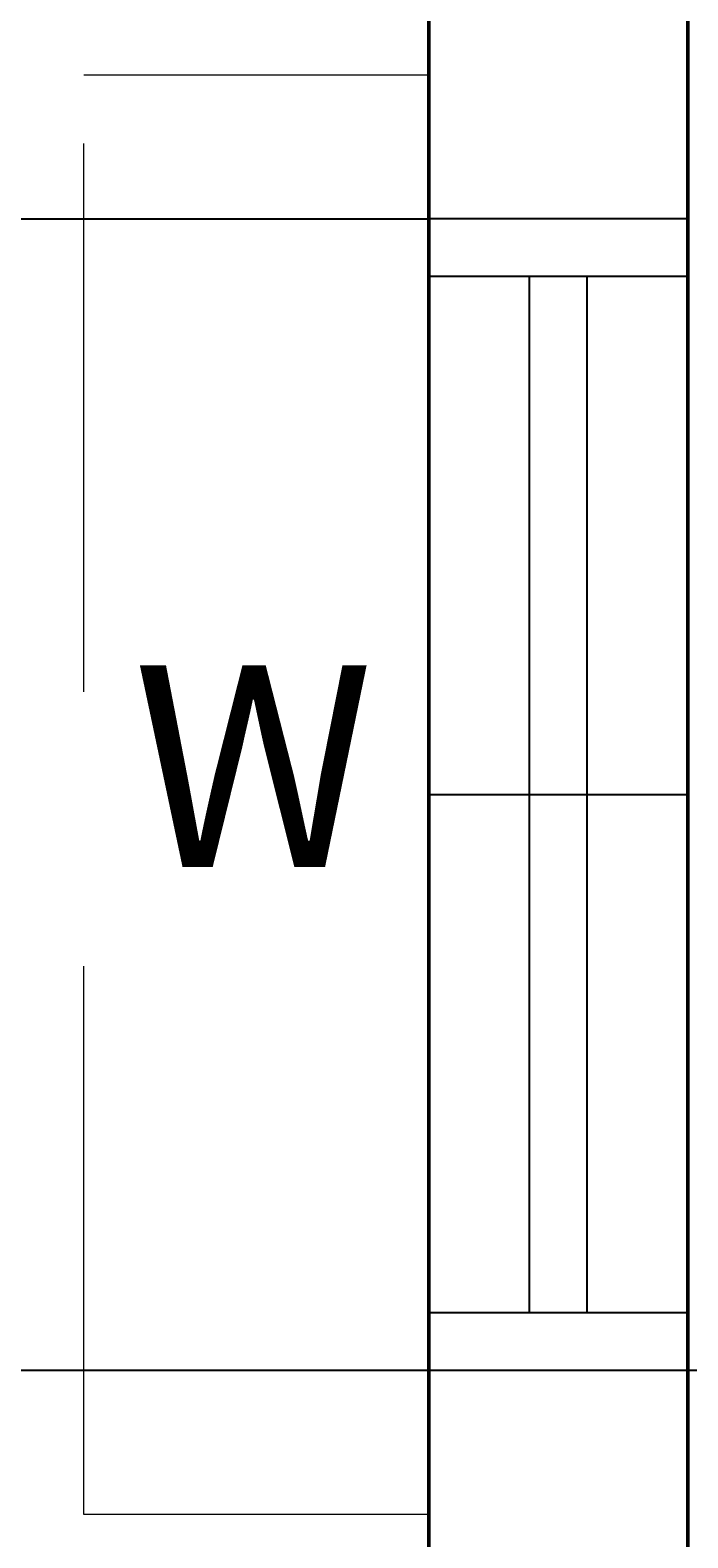
# Model space of a CAD drawing. Units: inches. Extents: x 37 to 824, y -700 to 234.
# Tile 51 of 77: x 147 to 170, y 107 to 160. Entities that reach past the tile are written whole.
import ezdxf

# ---------------------------------------------------------------- set-up
doc = ezdxf.new("R2010")
doc.units = ezdxf.units.IN
doc.header["$MEASUREMENT"] = 0
doc.linetypes.add('DASHED', pattern=[19.05, 12.7, -6.35])
for name, color, linetype, lineweight in [('A-ANNO-DIMS', 2, 'Continuous', 18), ('A-ANNO-TEXT', 7, 'Continuous', 18), ('A-GLAZ', 4, 'Continuous', 25), ('A-ROOF-OVHD', 1, 'DASHED', 18), ('A-WALL', 2, 'Continuous', 50)]:
    doc.layers.add(name, color=color, linetype=linetype, lineweight=lineweight)
doc.styles.get("Standard").update_dxf_attribs({"font": 'arial.ttf'})
doc.dimstyles.get("Standard").update_dxf_attribs({"dimtxt": 0.18, "dimasz": 0.18, "dimexe": 0.18, "dimexo": 0.0625, "dimgap": 0.09, "dimtad": 0, "dimtih": 1, "dimtoh": 1, "dimdec": 1, "dimzin": 0, "dimdsep": 46, "dimlunit": 4, "dimtxsty": 'Standard', "dimcen": 0.09, "dimadec": 0, "dimazin": 0, "dimtfac": 1, "dimtdec": 1, "dimtofl": 0, "dimtmove": 0, "dimatfit": 3, "dimfxl": 1, "dimtolj": 1, "dimtzin": 0, "dimarcsym": 0})

# ---------------------------------------------------------------- blocks, each defined once
blk = doc.blocks.new('WIN-900')
for p, q in [((0, 9), (0, 0)), ((2, 9), (2, 0)), ((20, 9), (20, 0)), ((38, 9), (38, 0)), ((40, 9), (40, 0)), ((38, 5.5), (2, 5.5)), ((38, 3.5), (2, 3.5))]:
    blk.add_line(p, q)
blk = doc.blocks.new('*D49')
at = {"layer": 'A-ANNO-DIMS', "color": 0, "lineweight": -2, "ltscale": 0.5, "transparency": 16777216}
for p, q in [((161.015, 191.09), (78.159, 191.09)), ((78.339, 190.91), (78.339, 172.272)), ((78.339, 153.27), (78.339, 171.908)), ((161.015, 153.09), (78.159, 153.09))]:
    blk.add_line(p, q, dxfattribs=at)
at = {"layer": 'A-ANNO-DIMS', "color": 0, "ltscale": 0.5, "transparency": 16777216}
for points in [[(78.309, 190.91), (78.369, 190.91), (78.339, 191.09)], [(78.309, 153.27), (78.369, 153.27), (78.339, 153.09)]]:
    blk.add_solid(points, dxfattribs=at)
at = {"layer": 'Defpoints', "color": 0, "ltscale": 0.5, "transparency": 16777216}
for p in [(161.077, 191.09), (78.339, 153.09), (161.077, 153.09)]:
    blk.add_point(p, dxfattribs=at)
at = {"layer": 'A-ANNO-DIMS', "color": 0, "ltscale": 0.5, "transparency": 16777216, "insert": (78.339, 172.09), "char_height": 0.18, "attachment_point": 5}
blk.add_mtext('\\A1;3\'-2"', dxfattribs=at)
blk = doc.blocks.new('*D50')
at = {"layer": 'A-ANNO-DIMS', "color": 0, "lineweight": -2, "ltscale": 0.5, "transparency": 16777216}
for p, q in [((161.015, 153.09), (78.159, 153.09)), ((78.339, 152.91), (78.339, 133.272)), ((78.339, 113.27), (78.339, 132.908)), ((161.015, 113.09), (78.159, 113.09))]:
    blk.add_line(p, q, dxfattribs=at)
at = {"layer": 'A-ANNO-DIMS', "color": 0, "ltscale": 0.5, "transparency": 16777216}
for points in [[(78.309, 152.91), (78.369, 152.91), (78.339, 153.09)], [(78.309, 113.27), (78.369, 113.27), (78.339, 113.09)]]:
    blk.add_solid(points, dxfattribs=at)
at = {"layer": 'Defpoints', "color": 0, "ltscale": 0.5, "transparency": 16777216}
for p in [(161.077, 153.09), (78.339, 113.09), (161.077, 113.09)]:
    blk.add_point(p, dxfattribs=at)
at = {"layer": 'A-ANNO-DIMS', "color": 0, "ltscale": 0.5, "transparency": 16777216, "insert": (78.339, 133.09), "char_height": 0.18, "attachment_point": 5}
blk.add_mtext('\\A1;3\'-4"', dxfattribs=at)
blk = doc.blocks.new('*D51')
at = {"layer": 'A-ANNO-DIMS', "color": 0, "lineweight": -2, "ltscale": 0.5, "transparency": 16777216}
for p, q in [((161.015, 113.09), (78.159, 113.09)), ((78.339, 112.91), (78.339, 81.772)), ((78.339, 50.27), (78.339, 81.408)), ((161.015, 50.09), (78.159, 50.09))]:
    blk.add_line(p, q, dxfattribs=at)
at = {"layer": 'A-ANNO-DIMS', "color": 0, "ltscale": 0.5, "transparency": 16777216}
for points in [[(78.309, 112.91), (78.369, 112.91), (78.339, 113.09)], [(78.309, 50.27), (78.369, 50.27), (78.339, 50.09)]]:
    blk.add_solid(points, dxfattribs=at)
at = {"layer": 'Defpoints', "color": 0, "ltscale": 0.5, "transparency": 16777216}
for p in [(161.077, 113.09), (78.339, 50.09), (161.077, 50.09)]:
    blk.add_point(p, dxfattribs=at)
at = {"layer": 'A-ANNO-DIMS', "color": 0, "ltscale": 0.5, "transparency": 16777216, "insert": (78.339, 81.59), "char_height": 0.18, "attachment_point": 5}
blk.add_mtext('\\A1;5\'-3"', dxfattribs=at)
blk = doc.blocks.new('*D60')
at = {"layer": 'A-ANNO-DIMS', "color": 0, "lineweight": -2, "ltscale": 0.5, "transparency": 16777216}
for p, q in [((419.015, 113.09), (78.159, 113.09)), ((78.339, 112.91), (78.339, 98.772)), ((78.339, 84.27), (78.339, 98.409)), ((419.015, 84.09), (78.159, 84.09))]:
    blk.add_line(p, q, dxfattribs=at)
at = {"layer": 'A-ANNO-DIMS', "color": 0, "ltscale": 0.5, "transparency": 16777216}
for points in [[(78.309, 112.91), (78.369, 112.91), (78.339, 113.09)], [(78.309, 84.27), (78.369, 84.27), (78.339, 84.09)]]:
    blk.add_solid(points, dxfattribs=at)
at = {"layer": 'Defpoints', "color": 0, "ltscale": 0.5, "transparency": 16777216}
for p in [(78.339, 113.09), (419.077, 113.09), (419.077, 84.09)]:
    blk.add_point(p, dxfattribs=at)
at = {"layer": 'A-ANNO-DIMS', "color": 0, "ltscale": 0.5, "transparency": 16777216, "insert": (78.339, 98.59), "char_height": 0.18, "attachment_point": 5}
blk.add_mtext('\\A1;2\'-5"', dxfattribs=at)

msp = doc.modelspace()

# ---------------------------------------------------------------- linework, layer by layer
at = {"layer": 'A-ROOF-OVHD', "ltscale": 1.5}
for p, q in [((161.077, 158.09), (149.077, 158.09)), ((149.077, 108.09), (149.077, 158.09)), ((161.077, 153.09), (161.077, 158.09)), ((161.077, 113.09), (161.077, 108.09)), ((161.077, 108.09), (149.077, 108.09))]:
    msp.add_line(p, q, dxfattribs=at)
at = {"layer": 'A-WALL'}
for p, q in [((161.077, 75.09), (161.077, 191.09)), ((170.077, 84.09), (170.077, 182.09))]:
    msp.add_line(p, q, dxfattribs=at)

# ---------------------------------------------------------------- block references
at = {"layer": 'A-GLAZ', "rotation": 269.9999999999999}
msp.add_blockref('WIN-900', (161.077, 153.091), dxfattribs=at)

# ---------------------------------------------------------------- texts
at = {"layer": 'A-ANNO-TEXT'}
msp.add_text('W', height=7, dxfattribs=at).set_placement((150.783, 130.582))

# ---------------------------------------------------------------- dimensions: what is measured, and where the dimension line sits
at = {"layer": 'A-ANNO-DIMS', "ltscale": 0.5}
for base, p1, p2, picture, middle in [((78.339, 153.09), (161.077, 191.09), (161.077, 153.09), '*D49', (78.339, 172.09)), ((78.339, 113.09), (161.077, 153.09), (161.077, 113.09), '*D50', (78.339, 133.09)), ((78.339, 50.09), (161.077, 113.09), (161.077, 50.09), '*D51', (78.339, 81.59)), ((78.339, 113.09), (419.077, 84.09), (419.077, 113.09), '*D60', (78.339, 98.59))]:
    dim = msp.add_linear_dim(base=base, p1=p1, p2=p2, angle=90, dimstyle='Standard', override={"dimdec": 1, "dimlfac": 1, "dimrnd": 0, "dimzin": 1, "dimdsep": 46, "dimlunit": 4, "dimfrac": 2}, dxfattribs=at)
    dim.commit()
    dim.dimension.update_dxf_attribs({"geometry": picture, "text_midpoint": middle})

doc.saveas('drawing.dxf')
